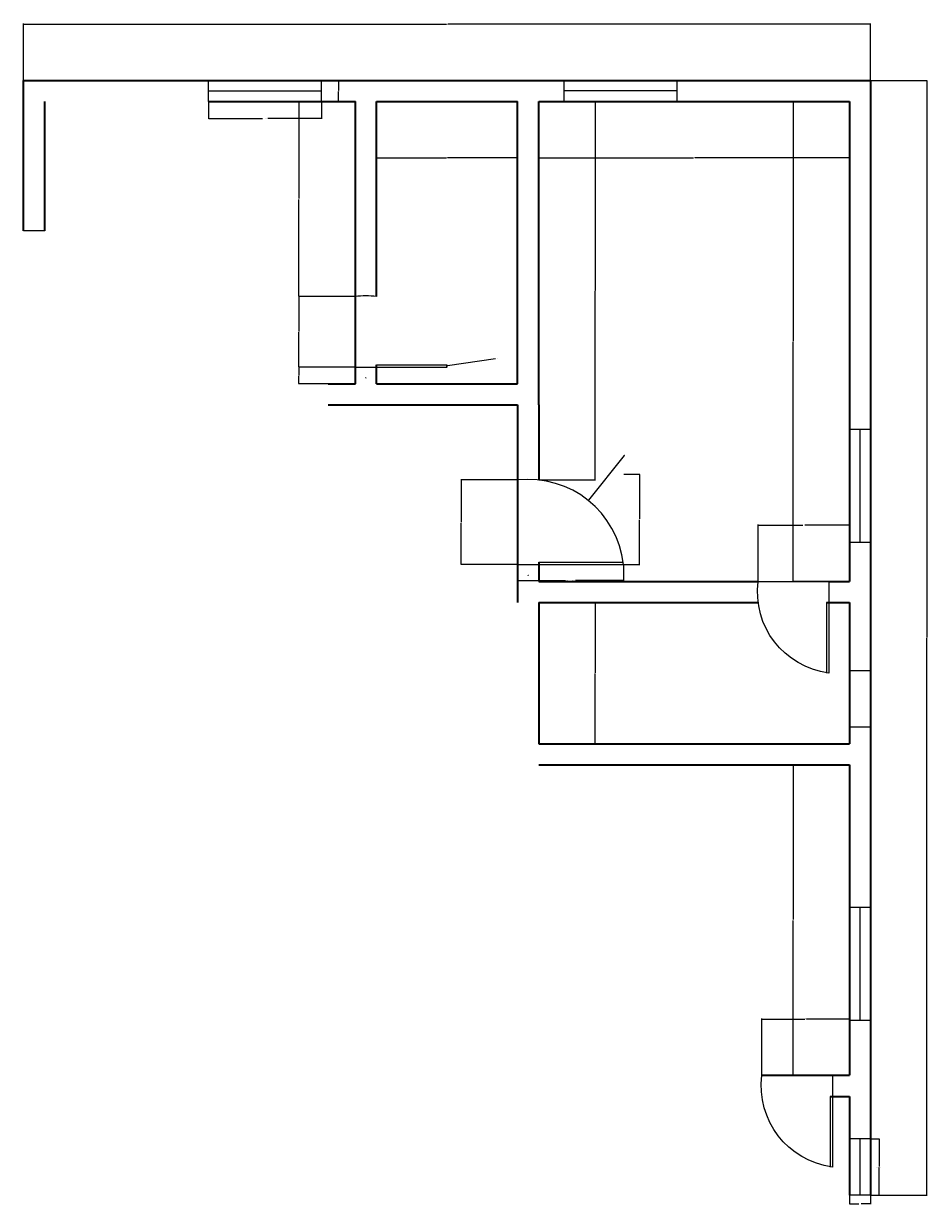
# Model space of a CAD drawing. Units: inches. Extents: x 4948 to 20975, y 6797 to 20508.
# Tile 2 of 5: x 14746 to 15130, y 6989 to 7491. Entities that reach past the tile are written whole.
import ezdxf

# ---------------------------------------------------------------- set-up
doc = ezdxf.new("R2010")
doc.units = ezdxf.units.IN
for name, color, linetype, lineweight in [('A-ANNO-DIMS', 2, 'Continuous', 18), ('A-DOOR', 3, 'Continuous', 18), ('A-GLAZ', 4, 'Continuous', 18), ('A-WALL', 7, 'Continuous', 35)]:
    doc.layers.add(name, color=color, linetype=linetype, lineweight=lineweight)
doc.styles.get("Standard").update_dxf_attribs({"font": 'times.ttf'})
doc.dimstyles.get("Standard").update_dxf_attribs({"dimtxt": 0.18, "dimasz": 0.18, "dimexe": 0.18, "dimexo": 0.0625, "dimgap": 0.09, "dimtad": 0, "dimtih": 1, "dimtoh": 1, "dimdec": 4, "dimzin": 0, "dimdsep": 46, "dimtxsty": 'Standard', "dimcen": 0.09, "dimadec": 0, "dimazin": 0, "dimtfac": 1, "dimtdec": 4, "dimtofl": 0, "dimtmove": 0, "dimatfit": 3, "dimfxl": 1, "dimtolj": 1, "dimtzin": 0, "dimarcsym": 0})

# ---------------------------------------------------------------- blocks, each defined once
blk = doc.blocks.new('DOOR-SINGLE-36IN')
for p, q in [((9, 1), (45, 1)), ((0, 0), (9, 0)), ((9, 0), (45, 0))]:
    blk.add_line(p, q)
blk.add_arc((4.5, -4.5), 40.75, 6.3402, 96.3402)
blk = doc.blocks.new('DOOR-SINGLE-30IN')
for p, q in [((0, 0), (9, 0)), ((9, 1), (39, 1)), ((9, 0), (39, 0))]:
    blk.add_line(p, q)
blk.add_arc((4.5, -4.5), 34.79, 7.4314, 97.4314)
blk = doc.blocks.new('WIN-48IN')
for p, q in [((0, 0), (0, 9)), ((48, 0), (48, 9)), ((0, 4.5), (48, 4.5))]:
    blk.add_line(p, q)
blk = doc.blocks.new('WIN-24IN')
for p, q in [((0, 24), (9, 24)), ((4.5, 0), (4.5, 24)), ((0, 0), (9, 0))]:
    blk.add_line(p, q)
blk = doc.blocks.new('*D9')
at = {"layer": 'A-ANNO-DIMS', "color": 0, "lineweight": -2, "transparency": 16777216}
for p, q in [((14824.47, 7457.38), (14824.47, 7450.06)), ((14872.47, 7457.38), (14872.47, 7450.06)), ((14824.65, 7450.24), (14847.33, 7450.24)), ((14872.29, 7450.24), (14849.62, 7450.24))]:
    blk.add_line(p, q, dxfattribs=at)
at = {"layer": 'A-ANNO-DIMS', "color": 0, "transparency": 16777216}
for points in [[(14824.65, 7450.27), (14824.65, 7450.21), (14824.47, 7450.24)], [(14872.29, 7450.27), (14872.29, 7450.21), (14872.47, 7450.24)]]:
    blk.add_solid(points, dxfattribs=at)
at = {"layer": 'Defpoints', "color": 0, "transparency": 16777216}
for p in [(14824.47, 7457.44), (14872.47, 7457.44), (14872.47, 7450.24)]:
    blk.add_point(p, dxfattribs=at)
at = {"layer": 'A-ANNO-DIMS', "color": 0, "transparency": 16777216, "insert": (14848.47, 7450.24), "char_height": 0.18, "attachment_point": 5}
blk.add_mtext('\\A1;WINDOW 48 TYP.', dxfattribs=at)
blk = doc.blocks.new('*D10')
at = {"layer": 'A-ANNO-DIMS', "color": 0, "lineweight": -2, "transparency": 16777216}
for p, q in [((14872.54, 7466.44), (14879.85, 7466.44)), ((14879.67, 7466.26), (14879.67, 7462.13)), ((14879.67, 7457.62), (14879.67, 7461.76)), ((14872.54, 7457.44), (14879.85, 7457.44))]:
    blk.add_line(p, q, dxfattribs=at)
at = {"layer": 'A-ANNO-DIMS', "color": 0, "transparency": 16777216}
for points in [[(14879.64, 7466.26), (14879.7, 7466.26), (14879.67, 7466.44)], [(14879.64, 7457.62), (14879.7, 7457.62), (14879.67, 7457.44)]]:
    blk.add_solid(points, dxfattribs=at)
at = {"layer": 'Defpoints', "color": 0, "transparency": 16777216}
for p in [(14872.47, 7466.44), (14879.67, 7466.44), (14872.47, 7457.44)]:
    blk.add_point(p, dxfattribs=at)
at = {"layer": 'A-ANNO-DIMS', "color": 0, "transparency": 16777216, "insert": (14879.67, 7461.94), "char_height": 0.18, "attachment_point": 5}
blk.add_mtext('\\A1;9 TYP.', dxfattribs=at)
blk = doc.blocks.new('*D13')
at = {"layer": 'A-ANNO-DIMS', "color": 0, "lineweight": -2, "transparency": 16777216}
for p, q in [((14955.85, 7260.49), (14955.85, 7253.62)), ((15000.85, 7260.49), (15000.85, 7253.62)), ((14956.03, 7253.8), (14976.25, 7253.8)), ((15000.67, 7253.8), (14980.46, 7253.8))]:
    blk.add_line(p, q, dxfattribs=at)
at = {"layer": 'A-ANNO-DIMS', "color": 0, "transparency": 16777216}
for points in [[(14956.03, 7253.83), (14956.03, 7253.77), (14955.85, 7253.8)], [(15000.67, 7253.83), (15000.67, 7253.77), (15000.85, 7253.8)]]:
    blk.add_solid(points, dxfattribs=at)
at = {"layer": 'Defpoints', "color": 0, "transparency": 16777216}
for p in [(14955.85, 7260.55), (15000.85, 7260.55), (15000.85, 7253.8)]:
    blk.add_point(p, dxfattribs=at)
at = {"layer": 'A-ANNO-DIMS', "color": 0, "transparency": 16777216, "insert": (14978.35, 7253.8), "char_height": 0.18, "attachment_point": 5}
blk.add_mtext('\\A1;BEDROOM DOOR SWING 45 TYP.', dxfattribs=at)
blk = doc.blocks.new('*D14')
at = {"layer": 'A-ANNO-DIMS', "color": 0, "lineweight": -2, "transparency": 16777216}
for p, q in [((15000.91, 7299.04), (15007.78, 7299.04)), ((15007.6, 7298.86), (15007.6, 7279.98)), ((15007.6, 7260.73), (15007.6, 7279.61)), ((15000.91, 7260.55), (15007.78, 7260.55))]:
    blk.add_line(p, q, dxfattribs=at)
at = {"layer": 'A-ANNO-DIMS', "color": 0, "transparency": 16777216}
for points in [[(15007.57, 7298.86), (15007.63, 7298.86), (15007.6, 7299.04)], [(15007.57, 7260.73), (15007.63, 7260.73), (15007.6, 7260.55)]]:
    blk.add_solid(points, dxfattribs=at)
at = {"layer": 'Defpoints', "color": 0, "transparency": 16777216}
for p in [(15000.85, 7299.04), (15007.6, 7299.04), (15000.85, 7260.55)]:
    blk.add_point(p, dxfattribs=at)
at = {"layer": 'A-ANNO-DIMS', "color": 0, "transparency": 16777216, "insert": (15007.6, 7279.8), "char_height": 0.18, "attachment_point": 5}
blk.add_mtext('\\A1;38 TYP.', dxfattribs=at)
blk = doc.blocks.new('*D15')
at = {"layer": 'A-ANNO-DIMS', "color": 0, "lineweight": -2, "transparency": 16777216}
for p, q in [((15105.91, 7016.44), (15109.63, 7016.44)), ((15109.45, 7016.26), (15109.45, 7004.63)), ((15109.45, 6992.62), (15109.45, 7004.26)), ((15105.91, 6992.44), (15109.63, 6992.44))]:
    blk.add_line(p, q, dxfattribs=at)
at = {"layer": 'A-ANNO-DIMS', "color": 0, "transparency": 16777216}
for points in [[(15109.42, 7016.26), (15109.48, 7016.26), (15109.45, 7016.44)], [(15109.42, 6992.62), (15109.48, 6992.62), (15109.45, 6992.44)]]:
    blk.add_solid(points, dxfattribs=at)
at = {"layer": 'Defpoints', "color": 0, "transparency": 16777216}
for p in [(15105.85, 7016.44), (15105.85, 6992.44), (15109.45, 6992.44)]:
    blk.add_point(p, dxfattribs=at)
at = {"layer": 'A-ANNO-DIMS', "color": 0, "transparency": 16777216, "insert": (15109.45, 7004.44), "char_height": 0.18, "attachment_point": 5}
blk.add_mtext('\\A1;TOILET WINDOW 24 TYP.', dxfattribs=at)
blk = doc.blocks.new('*D16')
at = {"layer": 'A-ANNO-DIMS', "color": 0, "lineweight": -2, "transparency": 16777216}
for p, q in [((15096.85, 6992.38), (15096.85, 6988.66)), ((15097.03, 6988.84), (15100.89, 6988.84)), ((15105.67, 6988.84), (15101.81, 6988.84)), ((15105.85, 6992.38), (15105.85, 6988.66))]:
    blk.add_line(p, q, dxfattribs=at)
at = {"layer": 'A-ANNO-DIMS', "color": 0, "transparency": 16777216}
for points in [[(15097.03, 6988.87), (15097.03, 6988.81), (15096.85, 6988.84)], [(15105.67, 6988.87), (15105.67, 6988.81), (15105.85, 6988.84)]]:
    blk.add_solid(points, dxfattribs=at)
at = {"layer": 'Defpoints', "color": 0, "transparency": 16777216}
for p in [(15096.85, 6992.44), (15096.85, 6988.84), (15105.85, 6992.44)]:
    blk.add_point(p, dxfattribs=at)
at = {"layer": 'A-ANNO-DIMS', "color": 0, "transparency": 16777216, "insert": (15101.35, 6988.84), "char_height": 0.18, "attachment_point": 5}
blk.add_mtext('\\A1;9 TYP.', dxfattribs=at)
blk = doc.blocks.new('*D73')
at = {"layer": 'A-ANNO-DIMS', "color": 0, "lineweight": -2, "transparency": 16777216}
for p, q in [((14745.85, 7466.51), (14745.85, 7490.57)), ((14746.03, 7490.39), (14925.57, 7490.39)), ((15105.67, 7490.39), (14926.13, 7490.39)), ((15105.85, 7466.51), (15105.85, 7490.57))]:
    blk.add_line(p, q, dxfattribs=at)
at = {"layer": 'A-ANNO-DIMS', "color": 0, "transparency": 16777216}
for points in [[(14746.03, 7490.42), (14746.03, 7490.36), (14745.85, 7490.39)], [(15105.67, 7490.42), (15105.67, 7490.36), (15105.85, 7490.39)]]:
    blk.add_solid(points, dxfattribs=at)
at = {"layer": 'Defpoints', "color": 0, "transparency": 16777216}
for p in [(15105.85, 7490.39), (14745.85, 7466.44), (15105.85, 7466.44)]:
    blk.add_point(p, dxfattribs=at)
at = {"layer": 'A-ANNO-DIMS', "color": 0, "transparency": 16777216, "insert": (14925.85, 7490.39), "char_height": 0.18, "attachment_point": 5}
blk.add_mtext('\\A1;360', dxfattribs=at)
blk = doc.blocks.new('*D74')
at = {"layer": 'A-ANNO-DIMS', "color": 0, "lineweight": -2, "transparency": 16777216}
for p, q in [((15105.91, 7466.44), (15129.98, 7466.44)), ((15129.8, 7466.26), (15129.8, 7229.63)), ((15129.8, 6992.62), (15129.8, 7229.26)), ((15105.91, 6992.44), (15129.98, 6992.44))]:
    blk.add_line(p, q, dxfattribs=at)
at = {"layer": 'A-ANNO-DIMS', "color": 0, "transparency": 16777216}
for points in [[(15129.77, 7466.26), (15129.83, 7466.26), (15129.8, 7466.44)], [(15129.77, 6992.62), (15129.83, 6992.62), (15129.8, 6992.44)]]:
    blk.add_solid(points, dxfattribs=at)
at = {"layer": 'Defpoints', "color": 0, "transparency": 16777216}
for p in [(15105.85, 7466.44), (15129.8, 7466.44), (15105.85, 6992.44)]:
    blk.add_point(p, dxfattribs=at)
at = {"layer": 'A-ANNO-DIMS', "color": 0, "transparency": 16777216, "insert": (15129.8, 7229.44), "char_height": 0.18, "attachment_point": 5}
blk.add_mtext('\\A1;474', dxfattribs=at)
blk = doc.blocks.new('*D75')
at = {"layer": 'A-ANNO-DIMS', "color": 0, "lineweight": -2, "transparency": 16777216}
for p, q in [((14895.85, 7457.38), (14895.85, 7433.31)), ((14955.85, 7457.38), (14955.85, 7433.31)), ((14896.03, 7433.49), (14925.64, 7433.49)), ((14955.67, 7433.49), (14926.06, 7433.49))]:
    blk.add_line(p, q, dxfattribs=at)
at = {"layer": 'A-ANNO-DIMS', "color": 0, "transparency": 16777216}
for points in [[(14896.03, 7433.52), (14896.03, 7433.46), (14895.85, 7433.49)], [(14955.67, 7433.52), (14955.67, 7433.46), (14955.85, 7433.49)]]:
    blk.add_solid(points, dxfattribs=at)
at = {"layer": 'Defpoints', "color": 0, "transparency": 16777216}
for p in [(14895.85, 7457.44), (14955.85, 7457.44), (14895.85, 7433.49)]:
    blk.add_point(p, dxfattribs=at)
at = {"layer": 'A-ANNO-DIMS', "color": 0, "transparency": 16777216, "insert": (14925.85, 7433.49), "char_height": 0.18, "attachment_point": 5}
blk.add_mtext('\\A1;60', dxfattribs=at)
blk = doc.blocks.new('*D76')
at = {"layer": 'A-ANNO-DIMS', "color": 0, "lineweight": -2, "transparency": 16777216}
for p, q in [((14964.85, 7457.38), (14964.85, 7433.31)), ((15096.85, 7457.38), (15096.85, 7433.31)), ((14965.03, 7433.49), (15030.58, 7433.49)), ((15096.67, 7433.49), (15031.12, 7433.49))]:
    blk.add_line(p, q, dxfattribs=at)
at = {"layer": 'A-ANNO-DIMS', "color": 0, "transparency": 16777216}
for points in [[(14965.03, 7433.52), (14965.03, 7433.46), (14964.85, 7433.49)], [(15096.67, 7433.52), (15096.67, 7433.46), (15096.85, 7433.49)]]:
    blk.add_solid(points, dxfattribs=at)
at = {"layer": 'Defpoints', "color": 0, "transparency": 16777216}
for p in [(14964.85, 7457.44), (15096.85, 7457.44), (14964.85, 7433.49)]:
    blk.add_point(p, dxfattribs=at)
at = {"layer": 'A-ANNO-DIMS', "color": 0, "transparency": 16777216, "insert": (15030.85, 7433.49), "char_height": 0.18, "attachment_point": 5}
blk.add_mtext('\\A1;132', dxfattribs=at)
blk = doc.blocks.new('*D77')
at = {"layer": 'A-ANNO-DIMS', "color": 0, "lineweight": -2, "transparency": 16777216}
for p, q in [((15096.79, 7457.44), (15072.72, 7457.44)), ((15072.9, 7457.26), (15072.9, 7355.63)), ((15072.9, 7253.62), (15072.9, 7355.26)), ((15096.79, 7253.44), (15072.72, 7253.44))]:
    blk.add_line(p, q, dxfattribs=at)
at = {"layer": 'A-ANNO-DIMS', "color": 0, "transparency": 16777216}
for points in [[(15072.87, 7457.26), (15072.93, 7457.26), (15072.9, 7457.44)], [(15072.87, 7253.62), (15072.93, 7253.62), (15072.9, 7253.44)]]:
    blk.add_solid(points, dxfattribs=at)
at = {"layer": 'Defpoints', "color": 0, "transparency": 16777216}
for p in [(15072.9, 7457.44), (15096.85, 7457.44), (15096.85, 7253.44)]:
    blk.add_point(p, dxfattribs=at)
at = {"layer": 'A-ANNO-DIMS', "color": 0, "transparency": 16777216, "insert": (15072.9, 7355.44), "char_height": 0.18, "attachment_point": 5}
blk.add_mtext('\\A1;204', dxfattribs=at)
blk = doc.blocks.new('*D78')
at = {"layer": 'A-ANNO-DIMS', "color": 0, "lineweight": -2, "transparency": 16777216}
for p, q in [((14964.91, 7244.44), (14988.98, 7244.44)), ((14988.8, 7244.26), (14988.8, 7214.63)), ((14988.8, 7184.62), (14988.8, 7214.26)), ((14964.91, 7184.44), (14988.98, 7184.44))]:
    blk.add_line(p, q, dxfattribs=at)
at = {"layer": 'A-ANNO-DIMS', "color": 0, "transparency": 16777216}
for points in [[(14988.77, 7244.26), (14988.83, 7244.26), (14988.8, 7244.44)], [(14988.77, 7184.62), (14988.83, 7184.62), (14988.8, 7184.44)]]:
    blk.add_solid(points, dxfattribs=at)
at = {"layer": 'Defpoints', "color": 0, "transparency": 16777216}
for p in [(14964.85, 7244.44), (14964.85, 7184.44), (14988.8, 7184.44)]:
    blk.add_point(p, dxfattribs=at)
at = {"layer": 'A-ANNO-DIMS', "color": 0, "transparency": 16777216, "insert": (14988.8, 7214.44), "char_height": 0.18, "attachment_point": 5}
blk.add_mtext('\\A1;60', dxfattribs=at)
blk = doc.blocks.new('*D79')
at = {"layer": 'A-ANNO-DIMS', "color": 0, "lineweight": -2, "transparency": 16777216}
for p, q in [((15096.79, 7175.44), (15072.72, 7175.44)), ((15072.9, 7175.26), (15072.9, 7109.63)), ((15072.9, 7043.62), (15072.9, 7109.26)), ((15096.79, 7043.44), (15072.72, 7043.44))]:
    blk.add_line(p, q, dxfattribs=at)
at = {"layer": 'A-ANNO-DIMS', "color": 0, "transparency": 16777216}
for points in [[(15072.87, 7175.26), (15072.93, 7175.26), (15072.9, 7175.44)], [(15072.87, 7043.62), (15072.93, 7043.62), (15072.9, 7043.44)]]:
    blk.add_solid(points, dxfattribs=at)
at = {"layer": 'Defpoints', "color": 0, "transparency": 16777216}
for p in [(15072.9, 7175.44), (15096.85, 7175.44), (15096.85, 7043.44)]:
    blk.add_point(p, dxfattribs=at)
at = {"layer": 'A-ANNO-DIMS', "color": 0, "transparency": 16777216, "insert": (15072.9, 7109.44), "char_height": 0.18, "attachment_point": 5}
blk.add_mtext('\\A1;132', dxfattribs=at)
blk = doc.blocks.new('*D80')
at = {"layer": 'A-ANNO-DIMS', "color": 0, "lineweight": -2, "transparency": 16777216}
for p, q in [((14886.79, 7457.44), (14862.72, 7457.44)), ((14862.9, 7457.26), (14862.9, 7416.16)), ((14862.9, 7374.69), (14862.9, 7415.79)), ((14886.79, 7374.51), (14862.72, 7374.51))]:
    blk.add_line(p, q, dxfattribs=at)
at = {"layer": 'A-ANNO-DIMS', "color": 0, "transparency": 16777216}
for points in [[(14862.87, 7457.26), (14862.93, 7457.26), (14862.9, 7457.44)], [(14862.87, 7374.69), (14862.93, 7374.69), (14862.9, 7374.51)]]:
    blk.add_solid(points, dxfattribs=at)
at = {"layer": 'Defpoints', "color": 0, "transparency": 16777216}
for p in [(14862.9, 7457.44), (14886.85, 7457.44), (14886.85, 7374.51)]:
    blk.add_point(p, dxfattribs=at)
at = {"layer": 'A-ANNO-DIMS', "color": 0, "transparency": 16777216, "insert": (14862.9, 7415.98), "char_height": 0.18, "attachment_point": 5}
blk.add_mtext('\\A1;82.93', dxfattribs=at)
blk = doc.blocks.new('*D81')
at = {"layer": 'A-ANNO-DIMS', "color": 0, "lineweight": -2, "transparency": 16777216}
for p, q in [((14886.79, 7374.51), (14862.72, 7374.51)), ((14862.9, 7374.33), (14862.9, 7359.69)), ((14862.9, 7344.69), (14862.9, 7359.33)), ((14886.79, 7344.51), (14862.72, 7344.51))]:
    blk.add_line(p, q, dxfattribs=at)
at = {"layer": 'A-ANNO-DIMS', "color": 0, "transparency": 16777216}
for points in [[(14862.87, 7374.33), (14862.93, 7374.33), (14862.9, 7374.51)], [(14862.87, 7344.69), (14862.93, 7344.69), (14862.9, 7344.51)]]:
    blk.add_solid(points, dxfattribs=at)
at = {"layer": 'Defpoints', "color": 0, "transparency": 16777216}
for p in [(14862.9, 7374.51), (14886.85, 7374.51), (14886.85, 7344.51)]:
    blk.add_point(p, dxfattribs=at)
at = {"layer": 'A-ANNO-DIMS', "color": 0, "transparency": 16777216, "insert": (14862.9, 7359.51), "char_height": 0.18, "attachment_point": 5}
blk.add_mtext('\\A1;30', dxfattribs=at)
blk = doc.blocks.new('*D82')
at = {"layer": 'A-ANNO-DIMS', "color": 0, "lineweight": -2, "transparency": 16777216}
for p, q in [((14886.79, 7344.51), (14862.72, 7344.51)), ((14862.9, 7344.33), (14862.9, 7341.16)), ((14862.9, 7337.62), (14862.9, 7340.79)), ((14886.79, 7337.44), (14862.72, 7337.44))]:
    blk.add_line(p, q, dxfattribs=at)
at = {"layer": 'A-ANNO-DIMS', "color": 0, "transparency": 16777216}
for points in [[(14862.87, 7344.33), (14862.93, 7344.33), (14862.9, 7344.51)], [(14862.87, 7337.62), (14862.93, 7337.62), (14862.9, 7337.44)]]:
    blk.add_solid(points, dxfattribs=at)
at = {"layer": 'Defpoints', "color": 0, "transparency": 16777216}
for p in [(14862.9, 7344.51), (14886.85, 7344.51), (14886.85, 7337.44)]:
    blk.add_point(p, dxfattribs=at)
at = {"layer": 'A-ANNO-DIMS', "color": 0, "transparency": 16777216, "insert": (14862.9, 7340.98), "char_height": 0.18, "attachment_point": 5}
blk.add_mtext('\\A1;7.065', dxfattribs=at)
blk = doc.blocks.new('*D83')
at = {"layer": 'A-ANNO-DIMS', "color": 0, "lineweight": -2, "transparency": 16777216}
for p, q in [((14964.91, 7457.44), (14988.98, 7457.44)), ((14988.8, 7457.26), (14988.8, 7377.18)), ((14988.8, 7296.73), (14988.8, 7376.82)), ((14964.91, 7296.55), (14988.98, 7296.55))]:
    blk.add_line(p, q, dxfattribs=at)
at = {"layer": 'A-ANNO-DIMS', "color": 0, "transparency": 16777216}
for points in [[(14988.77, 7457.26), (14988.83, 7457.26), (14988.8, 7457.44)], [(14988.77, 7296.73), (14988.83, 7296.73), (14988.8, 7296.55)]]:
    blk.add_solid(points, dxfattribs=at)
at = {"layer": 'Defpoints', "color": 0, "transparency": 16777216}
for p in [(14964.85, 7457.44), (14964.85, 7296.55), (14988.8, 7296.55)]:
    blk.add_point(p, dxfattribs=at)
at = {"layer": 'A-ANNO-DIMS', "color": 0, "transparency": 16777216, "insert": (14988.8, 7377), "char_height": 0.18, "attachment_point": 5}
blk.add_mtext('\\A1;160.9', dxfattribs=at)
blk = doc.blocks.new('*D84')
at = {"layer": 'A-ANNO-DIMS', "color": 0, "lineweight": -2, "transparency": 16777216}
for p, q in [((14955.79, 7296.55), (14931.72, 7296.55)), ((14931.9, 7296.37), (14931.9, 7278.73)), ((14931.9, 7260.73), (14931.9, 7278.37)), ((14955.79, 7260.55), (14931.72, 7260.55))]:
    blk.add_line(p, q, dxfattribs=at)
at = {"layer": 'A-ANNO-DIMS', "color": 0, "transparency": 16777216}
for points in [[(14931.87, 7296.37), (14931.93, 7296.37), (14931.9, 7296.55)], [(14931.87, 7260.73), (14931.93, 7260.73), (14931.9, 7260.55)]]:
    blk.add_solid(points, dxfattribs=at)
at = {"layer": 'Defpoints', "color": 0, "transparency": 16777216}
for p in [(14931.9, 7296.55), (14955.85, 7296.55), (14955.85, 7260.55)]:
    blk.add_point(p, dxfattribs=at)
at = {"layer": 'A-ANNO-DIMS', "color": 0, "transparency": 16777216, "insert": (14931.9, 7278.55), "char_height": 0.18, "attachment_point": 5}
blk.add_mtext('\\A1;36', dxfattribs=at)
blk = doc.blocks.new('*D85')
at = {"layer": 'A-ANNO-DIMS', "color": 0, "lineweight": -2, "transparency": 16777216}
for p, q in [((15058.09, 7253.51), (15058.09, 7277.57)), ((15058.27, 7277.39), (15077.09, 7277.39)), ((15096.67, 7277.39), (15077.85, 7277.39)), ((15096.85, 7253.51), (15096.85, 7277.57))]:
    blk.add_line(p, q, dxfattribs=at)
at = {"layer": 'A-ANNO-DIMS', "color": 0, "transparency": 16777216}
for points in [[(15058.27, 7277.42), (15058.27, 7277.36), (15058.09, 7277.39)], [(15096.67, 7277.42), (15096.67, 7277.36), (15096.85, 7277.39)]]:
    blk.add_solid(points, dxfattribs=at)
at = {"layer": 'Defpoints', "color": 0, "transparency": 16777216}
for p in [(15096.85, 7277.39), (15058.09, 7253.44), (15096.85, 7253.44)]:
    blk.add_point(p, dxfattribs=at)
at = {"layer": 'A-ANNO-DIMS', "color": 0, "transparency": 16777216, "insert": (15077.47, 7277.39), "char_height": 0.18, "attachment_point": 5}
blk.add_mtext('\\A1;38.76', dxfattribs=at)
blk = doc.blocks.new('*D86')
at = {"layer": 'A-ANNO-DIMS', "color": 0, "lineweight": -2, "transparency": 16777216}
for p, q in [((15059.69, 7043.51), (15059.69, 7067.57)), ((15059.87, 7067.39), (15077.89, 7067.39)), ((15096.67, 7067.39), (15078.65, 7067.39)), ((15096.85, 7043.51), (15096.85, 7067.57))]:
    blk.add_line(p, q, dxfattribs=at)
at = {"layer": 'A-ANNO-DIMS', "color": 0, "transparency": 16777216}
for points in [[(15059.87, 7067.42), (15059.87, 7067.36), (15059.69, 7067.39)], [(15096.67, 7067.42), (15096.67, 7067.36), (15096.85, 7067.39)]]:
    blk.add_solid(points, dxfattribs=at)
at = {"layer": 'Defpoints', "color": 0, "transparency": 16777216}
for p in [(15096.85, 7067.39), (15059.69, 7043.44), (15096.85, 7043.44)]:
    blk.add_point(p, dxfattribs=at)
at = {"layer": 'A-ANNO-DIMS', "color": 0, "transparency": 16777216, "insert": (15078.27, 7067.39), "char_height": 0.18, "attachment_point": 5}
blk.add_mtext('\\A1;37.16', dxfattribs=at)
blk = doc.blocks.new('*D96')
at = {"layer": 'A-ANNO-DIMS', "color": 0, "lineweight": -2, "transparency": 16777216}
for p, q in [((15001.08, 7306.96), (14985.92, 7288.01)), ((15001.26, 7306.96), (15001.08, 7306.96)), ((14960.26, 7256.05), (14960.44, 7256.05)), ((14960.35, 7255.96), (14960.35, 7256.14))]:
    blk.add_line(p, q, dxfattribs=at)
at = {"layer": 'A-ANNO-DIMS', "color": 0, "transparency": 16777216}
blk.add_solid([(14985.9, 7288.03), (14985.94, 7287.99), (14985.81, 7287.87)], dxfattribs=at)
at = {"layer": 'Defpoints', "color": 0, "transparency": 16777216}
for p in [(14985.81, 7287.87), (14960.35, 7256.05)]:
    blk.add_point(p, dxfattribs=at)
at = {"layer": 'A-ANNO-DIMS', "color": 0, "transparency": 16777216, "insert": (15001.73, 7306.96), "char_height": 0.18, "attachment_point": 5}
blk.add_mtext('\\A1;R40.75', dxfattribs=at)
blk = doc.blocks.new('*D97')
at = {"layer": 'A-ANNO-DIMS', "color": 0, "lineweight": -2, "transparency": 16777216}
for p, q in [((14946.44, 7348.01), (14925.96, 7345.04)), ((14891.26, 7340.01), (14891.44, 7340.01)), ((14891.35, 7339.92), (14891.35, 7340.1))]:
    blk.add_line(p, q, dxfattribs=at)
at = {"layer": 'A-ANNO-DIMS', "color": 0, "transparency": 16777216}
blk.add_solid([(14925.96, 7345.07), (14925.97, 7345.01), (14925.78, 7345.01)], dxfattribs=at)
at = {"layer": 'Defpoints', "color": 0, "transparency": 16777216}
for p in [(14925.78, 7345.01), (14891.35, 7340.01)]:
    blk.add_point(p, dxfattribs=at)
at = {"layer": 'A-ANNO-DIMS', "color": 0, "transparency": 16777216, "insert": (14947.11, 7348.01), "char_height": 0.18, "attachment_point": 5}
blk.add_mtext('\\A1;2X R34.79', dxfattribs=at)

msp = doc.modelspace()

# ---------------------------------------------------------------- linework, layer by layer
at = {"layer": 'A-DOOR'}
for p, q in [((14886.8522, 7344.5094), (14895.8522, 7344.5094)), ((14895.8522, 7345.5094), (14925.8522, 7345.5094)), ((14895.8522, 7344.5094), (14925.8522, 7344.5094)), ((15058.0899, 7253.444), (15088.0899, 7253.444))]:
    msp.add_line(p, q, dxfattribs=at)
for start, end in [(82.568592, 97.431408), (7.431408, 9.095541)]:
    msp.add_arc((14891.3522, 7340.0094), 34.7922, start, end, dxfattribs=at)
at = {"layer": 'A-GLAZ'}
for p, q in [((14754.8522, 7402.5352), (14745.8522, 7402.5352)), ((15096.8522, 7215.5422), (15105.8522, 7215.5422)), ((15096.8522, 7191.5422), (15105.8522, 7191.5422))]:
    msp.add_line(p, q, dxfattribs=at)
at = {"layer": 'A-WALL'}
for p, q in [((14745.8522, 7466.444), (15105.8522, 7466.444)), ((14745.8522, 7402.5352), (14745.8522, 7466.444)), ((15105.8522, 7466.444), (15105.8522, 6992.444)), ((14754.8522, 7402.5352), (14754.8522, 7457.444)), ((14824.4736, 7457.444), (14886.8522, 7457.444)), ((14886.8522, 7337.444), (14886.8522, 7457.444)), ((14895.8522, 7457.444), (14955.8522, 7457.444)), ((14895.8522, 7374.5094), (14895.8522, 7457.444)), ((14955.8522, 7337.444), (14955.8522, 7457.444)), ((14964.8522, 7457.444), (15096.8522, 7457.444)), ((14964.8522, 7328.444), (14964.8522, 7457.444)), ((15096.8522, 7457.444), (15096.8522, 7253.444)), ((14895.8522, 7337.444), (14895.8522, 7345.5094)), ((14875.3205, 7337.444), (14886.8522, 7337.444)), ((14895.8522, 7337.444), (14955.8522, 7337.444)), ((14875.3205, 7328.444), (14955.8522, 7328.444)), ((14955.8522, 7328.444), (14955.8522, 7244.444)), ((14964.8522, 7328.444), (14964.8522, 7296.5526)), ((14964.8522, 7261.5526), (14964.8522, 7253.444)), ((14964.8522, 7253.444), (15058.0899, 7253.444)), ((15088.0899, 7253.444), (15096.8522, 7253.444)), ((14964.8522, 7244.444), (15058.0899, 7244.444)), ((14964.8522, 7244.444), (14964.8522, 7184.444)), ((15087.0899, 7244.444), (15096.8522, 7244.444)), ((15096.8522, 7244.444), (15096.8522, 7184.444)), ((14964.8522, 7184.444), (15096.8522, 7184.444)), ((14964.8522, 7175.444), (15096.8522, 7175.444)), ((15096.8522, 7175.444), (15096.8522, 7043.444)), ((15059.6891, 7043.444), (15096.8522, 7043.444)), ((15088.6891, 7034.444), (15096.8522, 7034.444)), ((15096.8522, 7034.444), (15096.8522, 6992.444))]:
    msp.add_line(p, q, dxfattribs=at)

# ---------------------------------------------------------------- block references
at = {"layer": 'A-DOOR'}
msp.add_blockref('DOOR-SINGLE-36IN', (14955.8523, 7260.553), dxfattribs=at)
at = {"layer": 'A-DOOR', "extrusion": (0, 0, -1), "zscale": -1}
for p, rotation in [((-15088.0904, 7253.444), 269.9999999999977), ((-15089.6895, 7043.444), 269.9999999999877)]:
    msp.add_blockref('DOOR-SINGLE-30IN', p, dxfattribs=dict(at, rotation=rotation))
at = {"layer": 'A-GLAZ'}
msp.add_blockref('WIN-48IN', (14824.4733, 7457.444), dxfattribs=at)
for name, p, rotation in [('WIN-48IN', (15023.5125, 7466.4441), 180), ('WIN-48IN', (15096.8522, 7318.1491), 269.999999999967), ('WIN-48IN', (15096.8522, 7114.8958), 269.999999999993), ('WIN-24IN', (15105.8522, 7016.4442), 180)]:
    msp.add_blockref(name, p, dxfattribs=dict(at, rotation=rotation))

# ---------------------------------------------------------------- dimensions: what is measured, and where the dimension line sits
at = {"layer": 'A-ANNO-DIMS'}
for base, p1, p2, override, picture, middle in [((15105.8522, 7490.394), (14745.8522, 7466.444), (15105.8522, 7466.444), {"dimdec": 0, "dimlfac": 1, "dimrnd": 0, "dimzin": 0, "dimdsep": 46, "dimlunit": 2}, '*D73', (14925.8522, 7490.394)), ((15096.8522, 7277.394), (15058.0899, 7253.444), (15096.8522, 7253.444), {"dimdec": 2, "dimlfac": 1, "dimrnd": 0, "dimzin": 0, "dimdsep": 46, "dimlunit": 2}, '*D85', (15077.4711, 7277.394)), ((15096.8522, 7067.394), (15059.6891, 7043.444), (15096.8522, 7043.444), {"dimdec": 2, "dimlfac": 1, "dimrnd": 0, "dimzin": 0, "dimdsep": 46, "dimlunit": 2}, '*D86', (15078.2707, 7067.394))]:
    dim = msp.add_linear_dim(base=base, p1=p1, p2=p2, dimstyle='Standard', override=override, dxfattribs=at)
    dim.commit()
    dim.dimension.update_dxf_attribs({"geometry": picture, "text_midpoint": middle})
for base, p1, p2, angle, text, picture, middle in [((14879.6736, 7466.444), (14872.4736, 7457.444), (14872.4736, 7466.444), 90, '<> TYP.', '*D10', (14879.6736, 7461.944)), ((15007.6022, 7299.0379), (15000.8522, 7260.5526), (15000.8522, 7299.0379), 90, '<> TYP.', '*D14', (15007.6022, 7279.7953)), ((15109.4522, 6992.444), (15105.8522, 7016.444), (15105.8522, 6992.444), 270, 'TOILET WINDOW <> TYP.', '*D15', (15109.4522, 7004.444)), ((15096.8522, 6988.844), (15105.8522, 6992.444), (15096.8522, 6992.444), 180, '<> TYP.', '*D16', (15101.3522, 6988.844))]:
    dim = msp.add_linear_dim(base=base, p1=p1, p2=p2, angle=angle, text=text, dimstyle='Standard', override={"dimdec": 0, "dimlfac": 1, "dimrnd": 0, "dimzin": 0, "dimdsep": 46, "dimlunit": 2}, dxfattribs=at)
    dim.commit()
    dim.dimension.update_dxf_attribs({"geometry": picture, "text_midpoint": middle})
for base, p1, p2, angle, override, picture, middle in [((15129.8022, 7466.444), (15105.8522, 6992.444), (15105.8522, 7466.444), 90, {"dimdec": 0, "dimlfac": 1, "dimrnd": 0, "dimzin": 0, "dimdsep": 46, "dimlunit": 2}, '*D74', (15129.8022, 7229.444)), ((14862.9022, 7457.444), (14886.8522, 7374.5094), (14886.8522, 7457.444), 90, {"dimdec": 2, "dimlfac": 1, "dimrnd": 0, "dimzin": 0, "dimdsep": 46, "dimlunit": 2}, '*D80', (14862.9022, 7415.9767)), ((14895.8522, 7433.494), (14955.8522, 7457.444), (14895.8522, 7457.444), 180, {"dimdec": 0, "dimlfac": 1, "dimrnd": 0, "dimzin": 0, "dimdsep": 46, "dimlunit": 2}, '*D75', (14925.8522, 7433.494)), ((14964.8522, 7433.494), (15096.8522, 7457.444), (14964.8522, 7457.444), 180, {"dimdec": 0, "dimlfac": 1, "dimrnd": 0, "dimzin": 0, "dimdsep": 46, "dimlunit": 2}, '*D76', (15030.8522, 7433.494)), ((14988.8022, 7296.5526), (14964.8522, 7457.444), (14964.8522, 7296.5526), 270, {"dimdec": 1, "dimlfac": 1, "dimrnd": 0, "dimzin": 0, "dimdsep": 46, "dimlunit": 2}, '*D83', (14988.8022, 7376.9983)), ((15072.9022, 7457.444), (15096.8522, 7253.444), (15096.8522, 7457.444), 90, {"dimdec": 0, "dimlfac": 1, "dimrnd": 0, "dimzin": 0, "dimdsep": 46, "dimlunit": 2}, '*D77', (15072.9022, 7355.444)), ((14862.9022, 7374.5094), (14886.8522, 7344.5094), (14886.8522, 7374.5094), 90, {"dimdec": 0, "dimlfac": 1, "dimrnd": 0, "dimzin": 0, "dimdsep": 46, "dimlunit": 2}, '*D81', (14862.9022, 7359.5094)), ((14862.9022, 7344.5094), (14886.8522, 7337.444), (14886.8522, 7344.5094), 90, {"dimdec": 3, "dimlfac": 1, "dimrnd": 0, "dimzin": 0, "dimdsep": 46, "dimlunit": 2}, '*D82', (14862.9022, 7340.9767)), ((14931.9022, 7296.5526), (14955.8522, 7260.5526), (14955.8522, 7296.5526), 90, {"dimdec": 0, "dimlfac": 1, "dimrnd": 0, "dimzin": 0, "dimdsep": 46, "dimlunit": 2}, '*D84', (14931.9022, 7278.5526)), ((14988.8022, 7184.444), (14964.8522, 7244.444), (14964.8522, 7184.444), 270, {"dimdec": 0, "dimlfac": 1, "dimrnd": 0, "dimzin": 0, "dimdsep": 46, "dimlunit": 2}, '*D78', (14988.8022, 7214.444)), ((15072.9022, 7175.444), (15096.8522, 7043.444), (15096.8522, 7175.444), 90, {"dimdec": 0, "dimlfac": 1, "dimrnd": 0, "dimzin": 0, "dimdsep": 46, "dimlunit": 2}, '*D79', (15072.9022, 7109.444))]:
    dim = msp.add_linear_dim(base=base, p1=p1, p2=p2, angle=angle, dimstyle='Standard', override=override, dxfattribs=at)
    dim.commit()
    dim.dimension.update_dxf_attribs({"geometry": picture, "text_midpoint": middle})
for base, p1, p2, text, picture, middle in [((14872.4736, 7450.244), (14824.4736, 7457.444), (14872.4736, 7457.444), 'WINDOW <> TYP.', '*D9', (14848.4736, 7450.244)), ((15000.8522, 7253.8026), (14955.8522, 7260.5526), (15000.8522, 7260.5526), 'BEDROOM DOOR SWING <> TYP.', '*D13', (14978.3522, 7253.8026))]:
    dim = msp.add_linear_dim(base=base, p1=p1, p2=p2, text=text, dimstyle='Standard', override={"dimdec": 0, "dimlfac": 1, "dimrnd": 0, "dimzin": 0, "dimdsep": 46, "dimlunit": 2}, dxfattribs=at)
    dim.commit()
    dim.dimension.update_dxf_attribs({"geometry": picture, "text_midpoint": middle})
dim = msp.add_radius_dim(center=(14891.3522, 7340.0094), mpoint=(14925.7833, 7345.01), text='2X <>', dimstyle='Standard', override={"dimdec": 2, "dimlfac": 1, "dimrnd": 0, "dimzin": 0, "dimdsep": 46, "dimlunit": 2}, dxfattribs=at)
dim.commit()
dim.dimension.update_dxf_attribs({"geometry": '*D97', "text_midpoint": (14946.4419, 7348.0104), "dimtype": 164})
dim = msp.add_radius_dim(center=(14960.3522, 7256.0526), mpoint=(14985.8082, 7287.8723), dimstyle='Standard', override={"dimdec": 2, "dimlfac": 1, "dimrnd": 0, "dimzin": 0, "dimdsep": 46, "dimlunit": 2}, dxfattribs=at)
dim.commit()
dim.dimension.update_dxf_attribs({"geometry": '*D96', "text_midpoint": (15001.7285, 7306.9641), "dimtype": 164})

doc.saveas('drawing.dxf')
